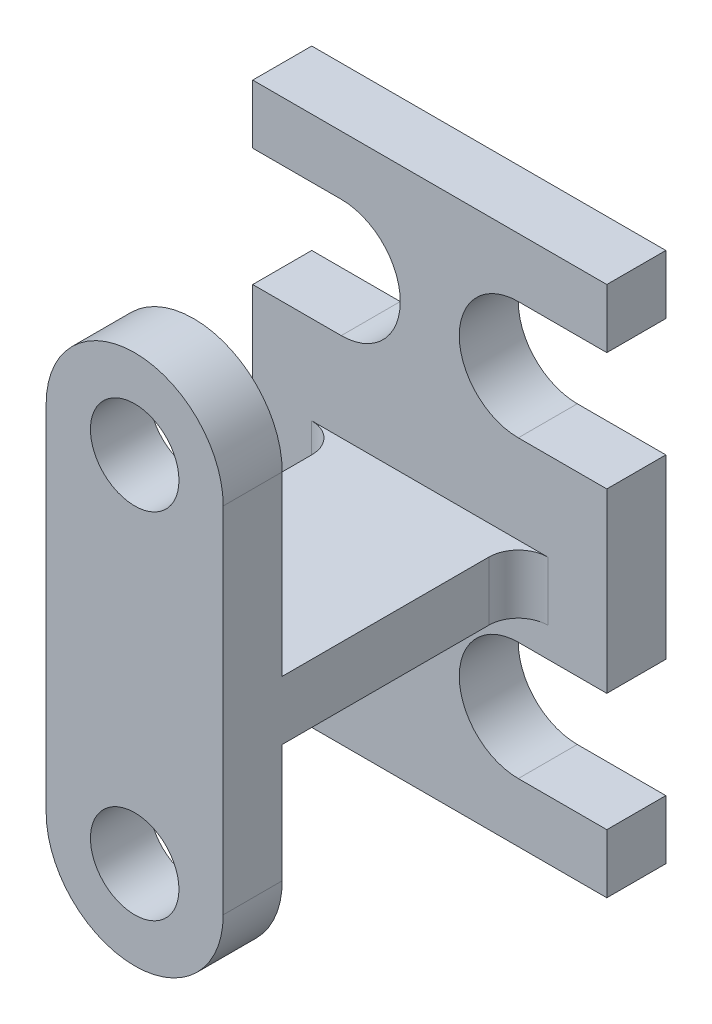
ISO-10303-21;
HEADER;
FILE_DESCRIPTION(('STEP AP214'),'2;1');
FILE_NAME('part.step','',(''),(''),'','','');
FILE_SCHEMA(('AUTOMOTIVE_DESIGN { 1 0 10303 214 1 1 1 1 }'));
ENDSEC;
DATA;
#1=APPLICATION_CONTEXT('core data for automotive mechanical design processes');
#2=APPLICATION_PROTOCOL_DEFINITION('international standard','automotive_design',2000,#1);
#3=PRODUCT_CONTEXT('',#1,'mechanical');
#4=PRODUCT('Part','Part','',(#3));
#5=PRODUCT_RELATED_PRODUCT_CATEGORY('part','',(#4));
#6=PRODUCT_DEFINITION_FORMATION('','',#4);
#7=PRODUCT_DEFINITION_CONTEXT('part definition',#1,'design');
#8=PRODUCT_DEFINITION('design','',#6,#7);
#9=PRODUCT_DEFINITION_SHAPE('','',#8);
#10=(LENGTH_UNIT() NAMED_UNIT(*) SI_UNIT(.MILLI.,.METRE.));
#11=(NAMED_UNIT(*) PLANE_ANGLE_UNIT() SI_UNIT($,.RADIAN.));
#12=(NAMED_UNIT(*) SI_UNIT($,.STERADIAN.) SOLID_ANGLE_UNIT());
#13=UNCERTAINTY_MEASURE_WITH_UNIT(LENGTH_MEASURE(1.E-05),#10,'distance_accuracy_value','');
#14=(GEOMETRIC_REPRESENTATION_CONTEXT(3) GLOBAL_UNCERTAINTY_ASSIGNED_CONTEXT((#13)) GLOBAL_UNIT_ASSIGNED_CONTEXT((#10,
#11,#12)) REPRESENTATION_CONTEXT('',''));
#15=CARTESIAN_POINT('',(0.,0.,0.));
#16=DIRECTION('',(0.,0.,1.));
#17=DIRECTION('',(1.,0.,0.));
#18=AXIS2_PLACEMENT_3D('',#15,#16,#17);
#19=CARTESIAN_POINT('',(0.,0.,0.));
#20=DIRECTION('',(0.,0.,1.));
#21=DIRECTION('',(1.,0.,0.));
#22=AXIS2_PLACEMENT_3D('',#19,#20,#21);
#23=PLANE('',#22);
#24=DIRECTION('',(1.,0.,0.));
#25=VECTOR('',#24,1.);
#26=CARTESIAN_POINT('',(-1.5,-3.5,0.));
#27=LINE('',#26,#25);
#28=CARTESIAN_POINT('',(-3.,-3.5,0.));
#29=VERTEX_POINT('',#28);
#30=CARTESIAN_POINT('',(-1.5,-3.5,0.));
#31=VERTEX_POINT('',#30);
#32=EDGE_CURVE('E327',#29,#31,#27,.T.);
#33=ORIENTED_EDGE('',*,*,#32,.F.);
#34=DIRECTION('',(0.,-1.,0.));
#35=VECTOR('',#34,1.);
#36=CARTESIAN_POINT('',(-3.,3.,0.));
#37=LINE('',#36,#35);
#38=CARTESIAN_POINT('',(-3.,-4.5,0.));
#39=VERTEX_POINT('',#38);
#40=EDGE_CURVE('E435',#29,#39,#37,.T.);
#41=ORIENTED_EDGE('',*,*,#40,.T.);
#42=DIRECTION('',(-1.,0.,0.));
#43=VECTOR('',#42,1.);
#44=CARTESIAN_POINT('',(-3.,-4.5,0.));
#45=LINE('',#44,#43);
#46=CARTESIAN_POINT('',(3.,-4.5,0.));
#47=VERTEX_POINT('',#46);
#48=EDGE_CURVE('E405',#47,#39,#45,.T.);
#49=ORIENTED_EDGE('',*,*,#48,.F.);
#50=DIRECTION('',(0.,1.,0.));
#51=VECTOR('',#50,1.);
#52=CARTESIAN_POINT('',(3.,3.,0.));
#53=LINE('',#52,#51);
#54=CARTESIAN_POINT('',(3.,-3.5,0.));
#55=VERTEX_POINT('',#54);
#56=EDGE_CURVE('E429',#47,#55,#53,.T.);
#57=ORIENTED_EDGE('',*,*,#56,.T.);
#58=DIRECTION('',(1.,0.,0.));
#59=VECTOR('',#58,1.);
#60=CARTESIAN_POINT('',(1.5,-3.5,0.));
#61=LINE('',#60,#59);
#62=CARTESIAN_POINT('',(1.5,-3.5,0.));
#63=VERTEX_POINT('',#62);
#64=EDGE_CURVE('E314',#63,#55,#61,.T.);
#65=ORIENTED_EDGE('',*,*,#64,.F.);
#66=CARTESIAN_POINT('',(1.5,-2.5,0.));
#67=DIRECTION('',(0.,0.,1.));
#68=DIRECTION('',(1.,0.,0.));
#69=AXIS2_PLACEMENT_3D('',#66,#67,#68);
#70=CIRCLE('',#69,1.);
#71=CARTESIAN_POINT('',(1.5,-1.5,0.));
#72=VERTEX_POINT('',#71);
#73=EDGE_CURVE('E311',#72,#63,#70,.T.);
#74=ORIENTED_EDGE('',*,*,#73,.F.);
#75=DIRECTION('',(-1.,0.,0.));
#76=VECTOR('',#75,1.);
#77=CARTESIAN_POINT('',(1.5,-1.5,0.));
#78=LINE('',#77,#76);
#79=CARTESIAN_POINT('',(3.,-1.5,0.));
#80=VERTEX_POINT('',#79);
#81=EDGE_CURVE('E307',#80,#72,#78,.T.);
#82=ORIENTED_EDGE('',*,*,#81,.F.);
#83=CARTESIAN_POINT('',(3.,1.5,0.));
#84=VERTEX_POINT('',#83);
#85=EDGE_CURVE('E433',#80,#84,#53,.T.);
#86=ORIENTED_EDGE('',*,*,#85,.T.);
#87=DIRECTION('',(1.,0.,0.));
#88=VECTOR('',#87,1.);
#89=CARTESIAN_POINT('',(1.5,1.5,0.));
#90=LINE('',#89,#88);
#91=CARTESIAN_POINT('',(1.5,1.5,0.));
#92=VERTEX_POINT('',#91);
#93=EDGE_CURVE('E292',#92,#84,#90,.T.);
#94=ORIENTED_EDGE('',*,*,#93,.F.);
#95=CARTESIAN_POINT('',(1.5,2.5,0.));
#96=DIRECTION('',(0.,0.,1.));
#97=DIRECTION('',(-1.,0.,0.));
#98=AXIS2_PLACEMENT_3D('',#95,#96,#97);
#99=CIRCLE('',#98,1.);
#100=CARTESIAN_POINT('',(1.5,3.5,0.));
#101=VERTEX_POINT('',#100);
#102=EDGE_CURVE('E287',#101,#92,#99,.T.);
#103=ORIENTED_EDGE('',*,*,#102,.F.);
#104=DIRECTION('',(-1.,0.,0.));
#105=VECTOR('',#104,1.);
#106=CARTESIAN_POINT('',(1.5,3.5,0.));
#107=LINE('',#106,#105);
#108=CARTESIAN_POINT('',(3.,3.5,0.));
#109=VERTEX_POINT('',#108);
#110=EDGE_CURVE('E294',#109,#101,#107,.T.);
#111=ORIENTED_EDGE('',*,*,#110,.F.);
#112=CARTESIAN_POINT('',(3.,4.5,0.));
#113=VERTEX_POINT('',#112);
#114=EDGE_CURVE('E416',#109,#113,#53,.T.);
#115=ORIENTED_EDGE('',*,*,#114,.T.);
#116=DIRECTION('',(1.,0.,0.));
#117=VECTOR('',#116,1.);
#118=CARTESIAN_POINT('',(-3.,4.5,0.));
#119=LINE('',#118,#117);
#120=CARTESIAN_POINT('',(-3.,4.5,0.));
#121=VERTEX_POINT('',#120);
#122=EDGE_CURVE('E409',#121,#113,#119,.T.);
#123=ORIENTED_EDGE('',*,*,#122,.F.);
#124=CARTESIAN_POINT('',(-3.,3.5,0.));
#125=VERTEX_POINT('',#124);
#126=EDGE_CURVE('E432',#121,#125,#37,.T.);
#127=ORIENTED_EDGE('',*,*,#126,.T.);
#128=DIRECTION('',(-1.,0.,0.));
#129=VECTOR('',#128,1.);
#130=CARTESIAN_POINT('',(-1.5,3.5,0.));
#131=LINE('',#130,#129);
#132=CARTESIAN_POINT('',(-1.5,3.5,0.));
#133=VERTEX_POINT('',#132);
#134=EDGE_CURVE('E345',#133,#125,#131,.T.);
#135=ORIENTED_EDGE('',*,*,#134,.F.);
#136=CARTESIAN_POINT('',(-1.5,2.5,0.));
#137=DIRECTION('',(0.,0.,1.));
#138=DIRECTION('',(1.,0.,0.));
#139=AXIS2_PLACEMENT_3D('',#136,#137,#138);
#140=CIRCLE('',#139,1.);
#141=CARTESIAN_POINT('',(-1.5,1.5,0.));
#142=VERTEX_POINT('',#141);
#143=EDGE_CURVE('E301',#142,#133,#140,.T.);
#144=ORIENTED_EDGE('',*,*,#143,.F.);
#145=DIRECTION('',(1.,0.,0.));
#146=VECTOR('',#145,1.);
#147=CARTESIAN_POINT('',(-1.5,1.5,0.));
#148=LINE('',#147,#146);
#149=CARTESIAN_POINT('',(-3.,1.5,0.));
#150=VERTEX_POINT('',#149);
#151=EDGE_CURVE('E341',#150,#142,#148,.T.);
#152=ORIENTED_EDGE('',*,*,#151,.F.);
#153=CARTESIAN_POINT('',(-3.,-1.5,0.));
#154=VERTEX_POINT('',#153);
#155=EDGE_CURVE('E440',#150,#154,#37,.T.);
#156=ORIENTED_EDGE('',*,*,#155,.T.);
#157=DIRECTION('',(-1.,0.,0.));
#158=VECTOR('',#157,1.);
#159=CARTESIAN_POINT('',(-1.5,-1.5,0.));
#160=LINE('',#159,#158);
#161=CARTESIAN_POINT('',(-1.5,-1.5,0.));
#162=VERTEX_POINT('',#161);
#163=EDGE_CURVE('E330',#162,#154,#160,.T.);
#164=ORIENTED_EDGE('',*,*,#163,.F.);
#165=CARTESIAN_POINT('',(-1.5,-2.5,0.));
#166=DIRECTION('',(0.,0.,1.));
#167=DIRECTION('',(-1.,0.,0.));
#168=AXIS2_PLACEMENT_3D('',#165,#166,#167);
#169=CIRCLE('',#168,1.);
#170=EDGE_CURVE('E288',#31,#162,#169,.T.);
#171=ORIENTED_EDGE('',*,*,#170,.F.);
#172=EDGE_LOOP('',(#33,#41,#49,#57,#65,#74,#82,#86,#94,#103,#111,#115,#123,#127,#135,#144,#152,
#156,#164,#171));
#173=FACE_BOUND('',#172,.T.);
#174=DIRECTION('',(1.,0.,0.));
#175=VECTOR('',#174,1.);
#176=CARTESIAN_POINT('',(1.5,-1.,0.));
#177=LINE('',#176,#175);
#178=CARTESIAN_POINT('',(-2.,-1.,0.));
#179=VERTEX_POINT('',#178);
#180=CARTESIAN_POINT('',(2.,-1.,0.));
#181=VERTEX_POINT('',#180);
#182=EDGE_CURVE('E57',#179,#181,#177,.T.);
#183=ORIENTED_EDGE('',*,*,#182,.F.);
#184=DIRECTION('',(0.,-1.,0.));
#185=VECTOR('',#184,1.);
#186=CARTESIAN_POINT('',(-2.,0.,0.));
#187=LINE('',#186,#185);
#188=CARTESIAN_POINT('',(-2.,0.,0.));
#189=VERTEX_POINT('',#188);
#190=EDGE_CURVE('E446',#179,#189,#187,.F.);
#191=ORIENTED_EDGE('',*,*,#190,.T.);
#192=DIRECTION('',(-1.,0.,0.));
#193=VECTOR('',#192,1.);
#194=CARTESIAN_POINT('',(-1.5,0.,0.));
#195=LINE('',#194,#193);
#196=CARTESIAN_POINT('',(2.,0.,0.));
#197=VERTEX_POINT('',#196);
#198=EDGE_CURVE('E64',#197,#189,#195,.T.);
#199=ORIENTED_EDGE('',*,*,#198,.F.);
#200=DIRECTION('',(0.,1.,0.));
#201=VECTOR('',#200,1.);
#202=CARTESIAN_POINT('',(2.,0.,0.));
#203=LINE('',#202,#201);
#204=EDGE_CURVE('E439',#197,#181,#203,.F.);
#205=ORIENTED_EDGE('',*,*,#204,.T.);
#206=EDGE_LOOP('',(#183,#191,#199,#205));
#207=FACE_BOUND('',#206,.T.);
#208=ADVANCED_FACE('F41',(#173,#207),#23,.T.);
#209=CARTESIAN_POINT('',(3.,3.,-1.));
#210=DIRECTION('',(1.,0.,0.));
#211=DIRECTION('',(0.,1.,0.));
#212=AXIS2_PLACEMENT_3D('',#209,#210,#211);
#213=PLANE('',#212);
#214=DIRECTION('',(0.,0.,1.));
#215=VECTOR('',#214,1.);
#216=CARTESIAN_POINT('',(3.,-1.5,-1.5));
#217=LINE('',#216,#215);
#218=CARTESIAN_POINT('',(3.,-1.5,-1.));
#219=VERTEX_POINT('',#218);
#220=EDGE_CURVE('E291',#219,#80,#217,.T.);
#221=ORIENTED_EDGE('',*,*,#220,.F.);
#222=DIRECTION('',(0.,1.,0.));
#223=VECTOR('',#222,1.);
#224=CARTESIAN_POINT('',(3.,3.,-1.));
#225=LINE('',#224,#223);
#226=CARTESIAN_POINT('',(3.,1.5,-1.));
#227=VERTEX_POINT('',#226);
#228=EDGE_CURVE('E422',#219,#227,#225,.T.);
#229=ORIENTED_EDGE('',*,*,#228,.T.);
#230=DIRECTION('',(0.,0.,1.));
#231=VECTOR('',#230,1.);
#232=CARTESIAN_POINT('',(3.,1.5,-1.5));
#233=LINE('',#232,#231);
#234=EDGE_CURVE('E302',#227,#84,#233,.T.);
#235=ORIENTED_EDGE('',*,*,#234,.T.);
#236=ORIENTED_EDGE('',*,*,#85,.F.);
#237=EDGE_LOOP('',(#221,#229,#235,#236));
#238=FACE_BOUND('',#237,.T.);
#239=ADVANCED_FACE('F503',(#238),#213,.T.);
#240=DIRECTION('',(0.,0.,1.));
#241=VECTOR('',#240,1.);
#242=CARTESIAN_POINT('',(3.,3.5,-1.5));
#243=LINE('',#242,#241);
#244=CARTESIAN_POINT('',(3.,3.5,-1.));
#245=VERTEX_POINT('',#244);
#246=EDGE_CURVE('E305',#245,#109,#243,.T.);
#247=ORIENTED_EDGE('',*,*,#246,.F.);
#248=CARTESIAN_POINT('',(3.,4.5,-1.));
#249=VERTEX_POINT('',#248);
#250=EDGE_CURVE('E421',#245,#249,#225,.T.);
#251=ORIENTED_EDGE('',*,*,#250,.T.);
#252=DIRECTION('',(0.,0.,-1.));
#253=VECTOR('',#252,1.);
#254=CARTESIAN_POINT('',(3.,4.5,-1.));
#255=LINE('',#254,#253);
#256=EDGE_CURVE('E411',#113,#249,#255,.T.);
#257=ORIENTED_EDGE('',*,*,#256,.F.);
#258=ORIENTED_EDGE('',*,*,#114,.F.);
#259=EDGE_LOOP('',(#247,#251,#257,#258));
#260=FACE_BOUND('',#259,.T.);
#261=ADVANCED_FACE('F509',(#260),#213,.T.);
#262=CARTESIAN_POINT('',(-3.,3.,-1.));
#263=DIRECTION('',(-1.,0.,0.));
#264=DIRECTION('',(0.,-1.,0.));
#265=AXIS2_PLACEMENT_3D('',#262,#263,#264);
#266=PLANE('',#265);
#267=DIRECTION('',(0.,0.,1.));
#268=VECTOR('',#267,1.);
#269=CARTESIAN_POINT('',(-3.,-3.5,-1.5));
#270=LINE('',#269,#268);
#271=CARTESIAN_POINT('',(-3.,-3.5,-1.));
#272=VERTEX_POINT('',#271);
#273=EDGE_CURVE('E333',#272,#29,#270,.T.);
#274=ORIENTED_EDGE('',*,*,#273,.F.);
#275=DIRECTION('',(0.,-1.,0.));
#276=VECTOR('',#275,1.);
#277=CARTESIAN_POINT('',(-3.,3.,-1.));
#278=LINE('',#277,#276);
#279=CARTESIAN_POINT('',(-3.,-4.5,-1.));
#280=VERTEX_POINT('',#279);
#281=EDGE_CURVE('E423',#272,#280,#278,.T.);
#282=ORIENTED_EDGE('',*,*,#281,.T.);
#283=DIRECTION('',(0.,0.,-1.));
#284=VECTOR('',#283,1.);
#285=CARTESIAN_POINT('',(-3.,-4.5,0.));
#286=LINE('',#285,#284);
#287=EDGE_CURVE('E393',#39,#280,#286,.T.);
#288=ORIENTED_EDGE('',*,*,#287,.F.);
#289=ORIENTED_EDGE('',*,*,#40,.F.);
#290=EDGE_LOOP('',(#274,#282,#288,#289));
#291=FACE_BOUND('',#290,.T.);
#292=ADVANCED_FACE('F525',(#291),#266,.T.);
#293=DIRECTION('',(0.,0.,1.));
#294=VECTOR('',#293,1.);
#295=CARTESIAN_POINT('',(-3.,-1.5,-1.5));
#296=LINE('',#295,#294);
#297=CARTESIAN_POINT('',(-3.,-1.5,-1.));
#298=VERTEX_POINT('',#297);
#299=EDGE_CURVE('E337',#298,#154,#296,.T.);
#300=ORIENTED_EDGE('',*,*,#299,.T.);
#301=ORIENTED_EDGE('',*,*,#155,.F.);
#302=DIRECTION('',(0.,0.,1.));
#303=VECTOR('',#302,1.);
#304=CARTESIAN_POINT('',(-3.,1.5,-1.5));
#305=LINE('',#304,#303);
#306=CARTESIAN_POINT('',(-3.,1.5,-1.));
#307=VERTEX_POINT('',#306);
#308=EDGE_CURVE('E354',#307,#150,#305,.T.);
#309=ORIENTED_EDGE('',*,*,#308,.F.);
#310=EDGE_CURVE('E426',#307,#298,#278,.T.);
#311=ORIENTED_EDGE('',*,*,#310,.T.);
#312=EDGE_LOOP('',(#300,#301,#309,#311));
#313=FACE_BOUND('',#312,.T.);
#314=ADVANCED_FACE('F523',(#313),#266,.T.);
#315=DIRECTION('',(0.,0.,1.));
#316=VECTOR('',#315,1.);
#317=CARTESIAN_POINT('',(3.,-3.5,-1.5));
#318=LINE('',#317,#316);
#319=CARTESIAN_POINT('',(3.,-3.5,-1.));
#320=VERTEX_POINT('',#319);
#321=EDGE_CURVE('E316',#320,#55,#318,.T.);
#322=ORIENTED_EDGE('',*,*,#321,.T.);
#323=ORIENTED_EDGE('',*,*,#56,.F.);
#324=DIRECTION('',(0.,0.,1.));
#325=VECTOR('',#324,1.);
#326=CARTESIAN_POINT('',(3.,-4.5,0.));
#327=LINE('',#326,#325);
#328=CARTESIAN_POINT('',(3.,-4.5,-1.));
#329=VERTEX_POINT('',#328);
#330=EDGE_CURVE('E398',#329,#47,#327,.T.);
#331=ORIENTED_EDGE('',*,*,#330,.F.);
#332=EDGE_CURVE('E420',#329,#320,#225,.T.);
#333=ORIENTED_EDGE('',*,*,#332,.T.);
#334=EDGE_LOOP('',(#322,#323,#331,#333));
#335=FACE_BOUND('',#334,.T.);
#336=ADVANCED_FACE('F514',(#335),#213,.T.);
#337=DIRECTION('',(0.,0.,1.));
#338=VECTOR('',#337,1.);
#339=CARTESIAN_POINT('',(-3.,3.5,-1.5));
#340=LINE('',#339,#338);
#341=CARTESIAN_POINT('',(-3.,3.5,-1.));
#342=VERTEX_POINT('',#341);
#343=EDGE_CURVE('E355',#342,#125,#340,.T.);
#344=ORIENTED_EDGE('',*,*,#343,.T.);
#345=ORIENTED_EDGE('',*,*,#126,.F.);
#346=DIRECTION('',(0.,0.,1.));
#347=VECTOR('',#346,1.);
#348=CARTESIAN_POINT('',(-3.,4.5,-1.));
#349=LINE('',#348,#347);
#350=CARTESIAN_POINT('',(-3.,4.5,-1.));
#351=VERTEX_POINT('',#350);
#352=EDGE_CURVE('E403',#351,#121,#349,.T.);
#353=ORIENTED_EDGE('',*,*,#352,.F.);
#354=EDGE_CURVE('E425',#351,#342,#278,.T.);
#355=ORIENTED_EDGE('',*,*,#354,.T.);
#356=EDGE_LOOP('',(#344,#345,#353,#355));
#357=FACE_BOUND('',#356,.T.);
#358=ADVANCED_FACE('F516',(#357),#266,.T.);
#359=CARTESIAN_POINT('',(0.,0.,-1.));
#360=DIRECTION('',(0.,0.,1.));
#361=DIRECTION('',(1.,0.,0.));
#362=AXIS2_PLACEMENT_3D('',#359,#360,#361);
#363=PLANE('',#362);
#364=ORIENTED_EDGE('',*,*,#281,.F.);
#365=DIRECTION('',(1.,0.,0.));
#366=VECTOR('',#365,1.);
#367=CARTESIAN_POINT('',(0.,-3.5,-1.));
#368=LINE('',#367,#366);
#369=CARTESIAN_POINT('',(-1.5,-3.5,-1.));
#370=VERTEX_POINT('',#369);
#371=EDGE_CURVE('E390',#272,#370,#368,.T.);
#372=ORIENTED_EDGE('',*,*,#371,.T.);
#373=CARTESIAN_POINT('',(-1.5,-2.5,-1.));
#374=DIRECTION('',(0.,0.,1.));
#375=DIRECTION('',(1.,0.,0.));
#376=AXIS2_PLACEMENT_3D('',#373,#374,#375);
#377=CIRCLE('',#376,1.);
#378=CARTESIAN_POINT('',(-1.5,-1.5,-1.));
#379=VERTEX_POINT('',#378);
#380=EDGE_CURVE('E388',#370,#379,#377,.T.);
#381=ORIENTED_EDGE('',*,*,#380,.T.);
#382=DIRECTION('',(-1.,0.,0.));
#383=VECTOR('',#382,1.);
#384=CARTESIAN_POINT('',(0.,-1.5,-1.));
#385=LINE('',#384,#383);
#386=EDGE_CURVE('E381',#379,#298,#385,.T.);
#387=ORIENTED_EDGE('',*,*,#386,.T.);
#388=ORIENTED_EDGE('',*,*,#310,.F.);
#389=DIRECTION('',(1.,0.,0.));
#390=VECTOR('',#389,1.);
#391=CARTESIAN_POINT('',(0.,1.5,-1.));
#392=LINE('',#391,#390);
#393=CARTESIAN_POINT('',(-1.5,1.5,-1.));
#394=VERTEX_POINT('',#393);
#395=EDGE_CURVE('E359',#307,#394,#392,.T.);
#396=ORIENTED_EDGE('',*,*,#395,.T.);
#397=CARTESIAN_POINT('',(-1.5,2.5,-1.));
#398=DIRECTION('',(0.,0.,1.));
#399=DIRECTION('',(1.,0.,0.));
#400=AXIS2_PLACEMENT_3D('',#397,#398,#399);
#401=CIRCLE('',#400,1.);
#402=CARTESIAN_POINT('',(-1.5,3.5,-1.));
#403=VERTEX_POINT('',#402);
#404=EDGE_CURVE('E361',#394,#403,#401,.T.);
#405=ORIENTED_EDGE('',*,*,#404,.T.);
#406=DIRECTION('',(-1.,0.,0.));
#407=VECTOR('',#406,1.);
#408=CARTESIAN_POINT('',(0.,3.5,-1.));
#409=LINE('',#408,#407);
#410=EDGE_CURVE('E349',#403,#342,#409,.T.);
#411=ORIENTED_EDGE('',*,*,#410,.T.);
#412=ORIENTED_EDGE('',*,*,#354,.F.);
#413=DIRECTION('',(-1.,0.,0.));
#414=VECTOR('',#413,1.);
#415=CARTESIAN_POINT('',(-3.,4.5,-1.));
#416=LINE('',#415,#414);
#417=EDGE_CURVE('E412',#249,#351,#416,.T.);
#418=ORIENTED_EDGE('',*,*,#417,.F.);
#419=ORIENTED_EDGE('',*,*,#250,.F.);
#420=DIRECTION('',(-1.,0.,0.));
#421=VECTOR('',#420,1.);
#422=CARTESIAN_POINT('',(0.,3.5,-1.));
#423=LINE('',#422,#421);
#424=CARTESIAN_POINT('',(1.5,3.5,-1.));
#425=VERTEX_POINT('',#424);
#426=EDGE_CURVE('E367',#245,#425,#423,.T.);
#427=ORIENTED_EDGE('',*,*,#426,.T.);
#428=CARTESIAN_POINT('',(1.5,2.5,-1.));
#429=DIRECTION('',(0.,0.,1.));
#430=DIRECTION('',(1.,0.,0.));
#431=AXIS2_PLACEMENT_3D('',#428,#429,#430);
#432=CIRCLE('',#431,1.);
#433=CARTESIAN_POINT('',(1.5,1.5,-1.));
#434=VERTEX_POINT('',#433);
#435=EDGE_CURVE('E375',#425,#434,#432,.T.);
#436=ORIENTED_EDGE('',*,*,#435,.T.);
#437=DIRECTION('',(1.,0.,0.));
#438=VECTOR('',#437,1.);
#439=CARTESIAN_POINT('',(0.,1.5,-1.));
#440=LINE('',#439,#438);
#441=EDGE_CURVE('E366',#434,#227,#440,.T.);
#442=ORIENTED_EDGE('',*,*,#441,.T.);
#443=ORIENTED_EDGE('',*,*,#228,.F.);
#444=DIRECTION('',(-1.,0.,0.));
#445=VECTOR('',#444,1.);
#446=CARTESIAN_POINT('',(0.,-1.5,-1.));
#447=LINE('',#446,#445);
#448=CARTESIAN_POINT('',(1.5,-1.5,-1.));
#449=VERTEX_POINT('',#448);
#450=EDGE_CURVE('E382',#219,#449,#447,.T.);
#451=ORIENTED_EDGE('',*,*,#450,.T.);
#452=CARTESIAN_POINT('',(1.5,-2.5,-1.));
#453=DIRECTION('',(0.,0.,1.));
#454=DIRECTION('',(1.,0.,0.));
#455=AXIS2_PLACEMENT_3D('',#452,#453,#454);
#456=CIRCLE('',#455,1.);
#457=CARTESIAN_POINT('',(1.5,-3.5,-1.));
#458=VERTEX_POINT('',#457);
#459=EDGE_CURVE('E374',#449,#458,#456,.T.);
#460=ORIENTED_EDGE('',*,*,#459,.T.);
#461=DIRECTION('',(1.,0.,0.));
#462=VECTOR('',#461,1.);
#463=CARTESIAN_POINT('',(0.,-3.5,-1.));
#464=LINE('',#463,#462);
#465=EDGE_CURVE('E377',#458,#320,#464,.T.);
#466=ORIENTED_EDGE('',*,*,#465,.T.);
#467=ORIENTED_EDGE('',*,*,#332,.F.);
#468=DIRECTION('',(1.,0.,0.));
#469=VECTOR('',#468,1.);
#470=CARTESIAN_POINT('',(-3.,-4.5,-1.));
#471=LINE('',#470,#469);
#472=EDGE_CURVE('E399',#280,#329,#471,.T.);
#473=ORIENTED_EDGE('',*,*,#472,.F.);
#474=EDGE_LOOP('',(#364,#372,#381,#387,#388,#396,#405,#411,#412,#418,#419,#427,#436,#442,#443,
#451,#460,#466,#467,#473));
#475=FACE_BOUND('',#474,.T.);
#476=ADVANCED_FACE('F520',(#475),#363,.F.);
#477=CARTESIAN_POINT('',(0.,4.5,0.));
#478=DIRECTION('',(0.,1.,0.));
#479=DIRECTION('',(0.,0.,1.));
#480=AXIS2_PLACEMENT_3D('',#477,#478,#479);
#481=PLANE('',#480);
#482=ORIENTED_EDGE('',*,*,#352,.T.);
#483=ORIENTED_EDGE('',*,*,#122,.T.);
#484=ORIENTED_EDGE('',*,*,#256,.T.);
#485=ORIENTED_EDGE('',*,*,#417,.T.);
#486=EDGE_LOOP('',(#482,#483,#484,#485));
#487=FACE_BOUND('',#486,.T.);
#488=ADVANCED_FACE('F587',(#487),#481,.T.);
#489=CARTESIAN_POINT('',(0.,-4.5,0.));
#490=DIRECTION('',(0.,-1.,0.));
#491=DIRECTION('',(0.,0.,-1.));
#492=AXIS2_PLACEMENT_3D('',#489,#490,#491);
#493=PLANE('',#492);
#494=ORIENTED_EDGE('',*,*,#287,.T.);
#495=ORIENTED_EDGE('',*,*,#472,.T.);
#496=ORIENTED_EDGE('',*,*,#330,.T.);
#497=ORIENTED_EDGE('',*,*,#48,.T.);
#498=EDGE_LOOP('',(#494,#495,#496,#497));
#499=FACE_BOUND('',#498,.T.);
#500=ADVANCED_FACE('F586',(#499),#493,.T.);
#501=CARTESIAN_POINT('',(-1.5,2.5,-1.5));
#502=DIRECTION('',(0.,0.,1.));
#503=DIRECTION('',(1.,0.,0.));
#504=AXIS2_PLACEMENT_3D('',#501,#502,#503);
#505=CYLINDRICAL_SURFACE('',#504,1.);
#506=DIRECTION('',(0.,0.,1.));
#507=VECTOR('',#506,1.);
#508=CARTESIAN_POINT('',(-1.5,1.5,-1.5));
#509=LINE('',#508,#507);
#510=EDGE_CURVE('E348',#394,#142,#509,.T.);
#511=ORIENTED_EDGE('',*,*,#510,.T.);
#512=ORIENTED_EDGE('',*,*,#143,.T.);
#513=DIRECTION('',(0.,0.,1.));
#514=VECTOR('',#513,1.);
#515=CARTESIAN_POINT('',(-1.5,3.5,-1.5));
#516=LINE('',#515,#514);
#517=EDGE_CURVE('E350',#403,#133,#516,.T.);
#518=ORIENTED_EDGE('',*,*,#517,.F.);
#519=ORIENTED_EDGE('',*,*,#404,.F.);
#520=EDGE_LOOP('',(#511,#512,#518,#519));
#521=FACE_BOUND('',#520,.T.);
#522=ADVANCED_FACE('F576',(#521),#505,.F.);
#523=CARTESIAN_POINT('',(-1.5,1.5,-1.5));
#524=DIRECTION('',(0.,-1.,0.));
#525=DIRECTION('',(1.,0.,0.));
#526=AXIS2_PLACEMENT_3D('',#523,#524,#525);
#527=PLANE('',#526);
#528=ORIENTED_EDGE('',*,*,#308,.T.);
#529=ORIENTED_EDGE('',*,*,#151,.T.);
#530=ORIENTED_EDGE('',*,*,#510,.F.);
#531=ORIENTED_EDGE('',*,*,#395,.F.);
#532=EDGE_LOOP('',(#528,#529,#530,#531));
#533=FACE_BOUND('',#532,.T.);
#534=ADVANCED_FACE('F577',(#533),#527,.F.);
#535=CARTESIAN_POINT('',(-1.5,3.5,-1.5));
#536=DIRECTION('',(0.,1.,0.));
#537=DIRECTION('',(-1.,0.,0.));
#538=AXIS2_PLACEMENT_3D('',#535,#536,#537);
#539=PLANE('',#538);
#540=ORIENTED_EDGE('',*,*,#517,.T.);
#541=ORIENTED_EDGE('',*,*,#134,.T.);
#542=ORIENTED_EDGE('',*,*,#343,.F.);
#543=ORIENTED_EDGE('',*,*,#410,.F.);
#544=EDGE_LOOP('',(#540,#541,#542,#543));
#545=FACE_BOUND('',#544,.T.);
#546=ADVANCED_FACE('F551',(#545),#539,.F.);
#547=CARTESIAN_POINT('',(1.5,2.5,-1.5));
#548=DIRECTION('',(0.,0.,1.));
#549=DIRECTION('',(1.,0.,0.));
#550=AXIS2_PLACEMENT_3D('',#547,#548,#549);
#551=CYLINDRICAL_SURFACE('',#550,1.);
#552=DIRECTION('',(0.,0.,1.));
#553=VECTOR('',#552,1.);
#554=CARTESIAN_POINT('',(1.5,3.5,-1.5));
#555=LINE('',#554,#553);
#556=EDGE_CURVE('E299',#425,#101,#555,.T.);
#557=ORIENTED_EDGE('',*,*,#556,.T.);
#558=ORIENTED_EDGE('',*,*,#102,.T.);
#559=DIRECTION('',(0.,0.,1.));
#560=VECTOR('',#559,1.);
#561=CARTESIAN_POINT('',(1.5,1.5,-1.5));
#562=LINE('',#561,#560);
#563=EDGE_CURVE('E296',#434,#92,#562,.T.);
#564=ORIENTED_EDGE('',*,*,#563,.F.);
#565=ORIENTED_EDGE('',*,*,#435,.F.);
#566=EDGE_LOOP('',(#557,#558,#564,#565));
#567=FACE_BOUND('',#566,.T.);
#568=ADVANCED_FACE('F544',(#567),#551,.F.);
#569=CARTESIAN_POINT('',(1.5,3.5,-1.5));
#570=DIRECTION('',(0.,1.,0.));
#571=DIRECTION('',(-1.,0.,0.));
#572=AXIS2_PLACEMENT_3D('',#569,#570,#571);
#573=PLANE('',#572);
#574=ORIENTED_EDGE('',*,*,#246,.T.);
#575=ORIENTED_EDGE('',*,*,#110,.T.);
#576=ORIENTED_EDGE('',*,*,#556,.F.);
#577=ORIENTED_EDGE('',*,*,#426,.F.);
#578=EDGE_LOOP('',(#574,#575,#576,#577));
#579=FACE_BOUND('',#578,.T.);
#580=ADVANCED_FACE('F541',(#579),#573,.F.);
#581=CARTESIAN_POINT('',(1.5,1.5,-1.5));
#582=DIRECTION('',(0.,-1.,0.));
#583=DIRECTION('',(1.,0.,0.));
#584=AXIS2_PLACEMENT_3D('',#581,#582,#583);
#585=PLANE('',#584);
#586=ORIENTED_EDGE('',*,*,#563,.T.);
#587=ORIENTED_EDGE('',*,*,#93,.T.);
#588=ORIENTED_EDGE('',*,*,#234,.F.);
#589=ORIENTED_EDGE('',*,*,#441,.F.);
#590=EDGE_LOOP('',(#586,#587,#588,#589));
#591=FACE_BOUND('',#590,.T.);
#592=ADVANCED_FACE('F542',(#591),#585,.F.);
#593=CARTESIAN_POINT('',(1.5,-1.5,-1.5));
#594=DIRECTION('',(0.,1.,0.));
#595=DIRECTION('',(-1.,0.,0.));
#596=AXIS2_PLACEMENT_3D('',#593,#594,#595);
#597=PLANE('',#596);
#598=ORIENTED_EDGE('',*,*,#220,.T.);
#599=ORIENTED_EDGE('',*,*,#81,.T.);
#600=DIRECTION('',(0.,0.,1.));
#601=VECTOR('',#600,1.);
#602=CARTESIAN_POINT('',(1.5,-1.5,-1.5));
#603=LINE('',#602,#601);
#604=EDGE_CURVE('E320',#449,#72,#603,.T.);
#605=ORIENTED_EDGE('',*,*,#604,.F.);
#606=ORIENTED_EDGE('',*,*,#450,.F.);
#607=EDGE_LOOP('',(#598,#599,#605,#606));
#608=FACE_BOUND('',#607,.T.);
#609=ADVANCED_FACE('F548',(#608),#597,.F.);
#610=CARTESIAN_POINT('',(1.5,-3.5,-1.5));
#611=DIRECTION('',(0.,-1.,0.));
#612=DIRECTION('',(1.,0.,0.));
#613=AXIS2_PLACEMENT_3D('',#610,#611,#612);
#614=PLANE('',#613);
#615=DIRECTION('',(0.,0.,1.));
#616=VECTOR('',#615,1.);
#617=CARTESIAN_POINT('',(1.5,-3.5,-1.5));
#618=LINE('',#617,#616);
#619=EDGE_CURVE('E325',#458,#63,#618,.T.);
#620=ORIENTED_EDGE('',*,*,#619,.T.);
#621=ORIENTED_EDGE('',*,*,#64,.T.);
#622=ORIENTED_EDGE('',*,*,#321,.F.);
#623=ORIENTED_EDGE('',*,*,#465,.F.);
#624=EDGE_LOOP('',(#620,#621,#622,#623));
#625=FACE_BOUND('',#624,.T.);
#626=ADVANCED_FACE('F554',(#625),#614,.F.);
#627=CARTESIAN_POINT('',(1.5,-2.5,-1.5));
#628=DIRECTION('',(0.,0.,1.));
#629=DIRECTION('',(1.,0.,0.));
#630=AXIS2_PLACEMENT_3D('',#627,#628,#629);
#631=CYLINDRICAL_SURFACE('',#630,1.);
#632=ORIENTED_EDGE('',*,*,#604,.T.);
#633=ORIENTED_EDGE('',*,*,#73,.T.);
#634=ORIENTED_EDGE('',*,*,#619,.F.);
#635=ORIENTED_EDGE('',*,*,#459,.F.);
#636=EDGE_LOOP('',(#632,#633,#634,#635));
#637=FACE_BOUND('',#636,.T.);
#638=ADVANCED_FACE('F556',(#637),#631,.F.);
#639=CARTESIAN_POINT('',(-1.5,-2.5,-1.5));
#640=DIRECTION('',(0.,0.,1.));
#641=DIRECTION('',(1.,0.,0.));
#642=AXIS2_PLACEMENT_3D('',#639,#640,#641);
#643=CYLINDRICAL_SURFACE('',#642,1.);
#644=DIRECTION('',(0.,0.,1.));
#645=VECTOR('',#644,1.);
#646=CARTESIAN_POINT('',(-1.5,-3.5,-1.5));
#647=LINE('',#646,#645);
#648=EDGE_CURVE('E315',#370,#31,#647,.T.);
#649=ORIENTED_EDGE('',*,*,#648,.T.);
#650=ORIENTED_EDGE('',*,*,#170,.T.);
#651=DIRECTION('',(0.,0.,1.));
#652=VECTOR('',#651,1.);
#653=CARTESIAN_POINT('',(-1.5,-1.5,-1.5));
#654=LINE('',#653,#652);
#655=EDGE_CURVE('E331',#379,#162,#654,.T.);
#656=ORIENTED_EDGE('',*,*,#655,.F.);
#657=ORIENTED_EDGE('',*,*,#380,.F.);
#658=EDGE_LOOP('',(#649,#650,#656,#657));
#659=FACE_BOUND('',#658,.T.);
#660=ADVANCED_FACE('F565',(#659),#643,.F.);
#661=CARTESIAN_POINT('',(-1.5,-3.5,-1.5));
#662=DIRECTION('',(0.,-1.,0.));
#663=DIRECTION('',(1.,0.,0.));
#664=AXIS2_PLACEMENT_3D('',#661,#662,#663);
#665=PLANE('',#664);
#666=ORIENTED_EDGE('',*,*,#273,.T.);
#667=ORIENTED_EDGE('',*,*,#32,.T.);
#668=ORIENTED_EDGE('',*,*,#648,.F.);
#669=ORIENTED_EDGE('',*,*,#371,.F.);
#670=EDGE_LOOP('',(#666,#667,#668,#669));
#671=FACE_BOUND('',#670,.T.);
#672=ADVANCED_FACE('F570',(#671),#665,.F.);
#673=CARTESIAN_POINT('',(-1.5,-1.5,-1.5));
#674=DIRECTION('',(0.,1.,0.));
#675=DIRECTION('',(-1.,0.,0.));
#676=AXIS2_PLACEMENT_3D('',#673,#674,#675);
#677=PLANE('',#676);
#678=ORIENTED_EDGE('',*,*,#655,.T.);
#679=ORIENTED_EDGE('',*,*,#163,.T.);
#680=ORIENTED_EDGE('',*,*,#299,.F.);
#681=ORIENTED_EDGE('',*,*,#386,.F.);
#682=EDGE_LOOP('',(#678,#679,#680,#681));
#683=FACE_BOUND('',#682,.T.);
#684=ADVANCED_FACE('F538',(#683),#677,.F.);
#685=CARTESIAN_POINT('',(1.5,-1.,4.));
#686=DIRECTION('',(0.,1.,0.));
#687=DIRECTION('',(0.,0.,1.));
#688=AXIS2_PLACEMENT_3D('',#685,#686,#687);
#689=PLANE('',#688);
#690=ORIENTED_EDGE('',*,*,#182,.T.);
#691=CARTESIAN_POINT('',(2.,-1.,0.5));
#692=DIRECTION('',(0.,1.,0.));
#693=DIRECTION('',(0.,0.,1.));
#694=AXIS2_PLACEMENT_3D('',#691,#692,#693);
#695=CIRCLE('',#694,0.5);
#696=CARTESIAN_POINT('',(1.5,-1.,0.5));
#697=VERTEX_POINT('',#696);
#698=EDGE_CURVE('E443',#181,#697,#695,.T.);
#699=ORIENTED_EDGE('',*,*,#698,.T.);
#700=DIRECTION('',(0.,0.,-1.));
#701=VECTOR('',#700,1.);
#702=CARTESIAN_POINT('',(1.5,-1.,4.));
#703=LINE('',#702,#701);
#704=CARTESIAN_POINT('',(1.5,-1.,4.));
#705=VERTEX_POINT('',#704);
#706=EDGE_CURVE('E289',#705,#697,#703,.T.);
#707=ORIENTED_EDGE('',*,*,#706,.F.);
#708=DIRECTION('',(1.,0.,0.));
#709=VECTOR('',#708,1.);
#710=CARTESIAN_POINT('',(1.5,-1.,4.));
#711=LINE('',#710,#709);
#712=CARTESIAN_POINT('',(-1.5,-1.,4.));
#713=VERTEX_POINT('',#712);
#714=EDGE_CURVE('E272',#713,#705,#711,.T.);
#715=ORIENTED_EDGE('',*,*,#714,.F.);
#716=DIRECTION('',(0.,0.,-1.));
#717=VECTOR('',#716,1.);
#718=CARTESIAN_POINT('',(-1.5,-1.,4.));
#719=LINE('',#718,#717);
#720=CARTESIAN_POINT('',(-1.5,-1.,0.5));
#721=VERTEX_POINT('',#720);
#722=EDGE_CURVE('E277',#713,#721,#719,.T.);
#723=ORIENTED_EDGE('',*,*,#722,.T.);
#724=CARTESIAN_POINT('',(-2.,-1.,0.5));
#725=DIRECTION('',(0.,1.,0.));
#726=DIRECTION('',(0.,0.,1.));
#727=AXIS2_PLACEMENT_3D('',#724,#725,#726);
#728=CIRCLE('',#727,0.5);
#729=EDGE_CURVE('E47',#721,#179,#728,.T.);
#730=ORIENTED_EDGE('',*,*,#729,.T.);
#731=EDGE_LOOP('',(#690,#699,#707,#715,#723,#730));
#732=FACE_BOUND('',#731,.T.);
#733=ADVANCED_FACE('F455',(#732),#689,.F.);
#734=CARTESIAN_POINT('',(1.5,0.,4.));
#735=DIRECTION('',(-1.,0.,0.));
#736=DIRECTION('',(0.,0.,1.));
#737=AXIS2_PLACEMENT_3D('',#734,#735,#736);
#738=PLANE('',#737);
#739=ORIENTED_EDGE('',*,*,#706,.T.);
#740=DIRECTION('',(0.,1.,0.));
#741=VECTOR('',#740,1.);
#742=CARTESIAN_POINT('',(1.5,0.,0.5));
#743=LINE('',#742,#741);
#744=CARTESIAN_POINT('',(1.5,0.,0.5));
#745=VERTEX_POINT('',#744);
#746=EDGE_CURVE('E430',#697,#745,#743,.T.);
#747=ORIENTED_EDGE('',*,*,#746,.T.);
#748=DIRECTION('',(0.,0.,-1.));
#749=VECTOR('',#748,1.);
#750=CARTESIAN_POINT('',(1.5,0.,4.));
#751=LINE('',#750,#749);
#752=CARTESIAN_POINT('',(1.5,0.,4.));
#753=VERTEX_POINT('',#752);
#754=EDGE_CURVE('E283',#753,#745,#751,.T.);
#755=ORIENTED_EDGE('',*,*,#754,.F.);
#756=DIRECTION('',(0.,1.,0.));
#757=VECTOR('',#756,1.);
#758=CARTESIAN_POINT('',(1.5,3.,4.));
#759=LINE('',#758,#757);
#760=CARTESIAN_POINT('',(1.5,3.,4.));
#761=VERTEX_POINT('',#760);
#762=EDGE_CURVE('E475',#753,#761,#759,.T.);
#763=ORIENTED_EDGE('',*,*,#762,.T.);
#764=DIRECTION('',(0.,0.,-1.));
#765=VECTOR('',#764,1.);
#766=CARTESIAN_POINT('',(1.5,3.,5.));
#767=LINE('',#766,#765);
#768=CARTESIAN_POINT('',(1.5,3.,5.));
#769=VERTEX_POINT('',#768);
#770=EDGE_CURVE('E478',#769,#761,#767,.T.);
#771=ORIENTED_EDGE('',*,*,#770,.F.);
#772=DIRECTION('',(0.,1.,0.));
#773=VECTOR('',#772,1.);
#774=CARTESIAN_POINT('',(1.5,3.,5.));
#775=LINE('',#774,#773);
#776=CARTESIAN_POINT('',(1.5,-3.,5.));
#777=VERTEX_POINT('',#776);
#778=EDGE_CURVE('E257',#777,#769,#775,.T.);
#779=ORIENTED_EDGE('',*,*,#778,.F.);
#780=DIRECTION('',(0.,0.,-1.));
#781=VECTOR('',#780,1.);
#782=CARTESIAN_POINT('',(1.5,-3.,5.));
#783=LINE('',#782,#781);
#784=CARTESIAN_POINT('',(1.5,-3.,4.));
#785=VERTEX_POINT('',#784);
#786=EDGE_CURVE('E266',#777,#785,#783,.T.);
#787=ORIENTED_EDGE('',*,*,#786,.T.);
#788=EDGE_CURVE('E258',#785,#705,#759,.T.);
#789=ORIENTED_EDGE('',*,*,#788,.T.);
#790=EDGE_LOOP('',(#739,#747,#755,#763,#771,#779,#787,#789));
#791=FACE_BOUND('',#790,.T.);
#792=ADVANCED_FACE('F467',(#791),#738,.F.);
#793=CARTESIAN_POINT('',(-1.5,0.,4.));
#794=DIRECTION('',(0.,-1.,0.));
#795=DIRECTION('',(0.,0.,-1.));
#796=AXIS2_PLACEMENT_3D('',#793,#794,#795);
#797=PLANE('',#796);
#798=ORIENTED_EDGE('',*,*,#198,.T.);
#799=CARTESIAN_POINT('',(-2.,0.,0.5));
#800=DIRECTION('',(0.,-1.,0.));
#801=DIRECTION('',(0.,0.,-1.));
#802=AXIS2_PLACEMENT_3D('',#799,#800,#801);
#803=CIRCLE('',#802,0.5);
#804=CARTESIAN_POINT('',(-1.5,0.,0.5));
#805=VERTEX_POINT('',#804);
#806=EDGE_CURVE('E11',#189,#805,#803,.T.);
#807=ORIENTED_EDGE('',*,*,#806,.T.);
#808=DIRECTION('',(0.,0.,-1.));
#809=VECTOR('',#808,1.);
#810=CARTESIAN_POINT('',(-1.5,0.,4.));
#811=LINE('',#810,#809);
#812=CARTESIAN_POINT('',(-1.5,0.,4.));
#813=VERTEX_POINT('',#812);
#814=EDGE_CURVE('E281',#813,#805,#811,.T.);
#815=ORIENTED_EDGE('',*,*,#814,.F.);
#816=DIRECTION('',(-1.,0.,0.));
#817=VECTOR('',#816,1.);
#818=CARTESIAN_POINT('',(-1.5,0.,4.));
#819=LINE('',#818,#817);
#820=EDGE_CURVE('E274',#753,#813,#819,.T.);
#821=ORIENTED_EDGE('',*,*,#820,.F.);
#822=ORIENTED_EDGE('',*,*,#754,.T.);
#823=CARTESIAN_POINT('',(2.,0.,0.5));
#824=DIRECTION('',(0.,-1.,0.));
#825=DIRECTION('',(0.,0.,-1.));
#826=AXIS2_PLACEMENT_3D('',#823,#824,#825);
#827=CIRCLE('',#826,0.5);
#828=EDGE_CURVE('E445',#745,#197,#827,.T.);
#829=ORIENTED_EDGE('',*,*,#828,.T.);
#830=EDGE_LOOP('',(#798,#807,#815,#821,#822,#829));
#831=FACE_BOUND('',#830,.T.);
#832=ADVANCED_FACE('F457',(#831),#797,.F.);
#833=CARTESIAN_POINT('',(-1.5,-1.,4.));
#834=DIRECTION('',(1.,0.,0.));
#835=DIRECTION('',(0.,0.,-1.));
#836=AXIS2_PLACEMENT_3D('',#833,#834,#835);
#837=PLANE('',#836);
#838=ORIENTED_EDGE('',*,*,#814,.T.);
#839=DIRECTION('',(0.,-1.,0.));
#840=VECTOR('',#839,1.);
#841=CARTESIAN_POINT('',(-1.5,-1.,0.5));
#842=LINE('',#841,#840);
#843=EDGE_CURVE('E447',#805,#721,#842,.T.);
#844=ORIENTED_EDGE('',*,*,#843,.T.);
#845=ORIENTED_EDGE('',*,*,#722,.F.);
#846=DIRECTION('',(0.,-1.,0.));
#847=VECTOR('',#846,1.);
#848=CARTESIAN_POINT('',(-1.5,3.,4.));
#849=LINE('',#848,#847);
#850=CARTESIAN_POINT('',(-1.5,-3.,4.));
#851=VERTEX_POINT('',#850);
#852=EDGE_CURVE('E481',#713,#851,#849,.T.);
#853=ORIENTED_EDGE('',*,*,#852,.T.);
#854=DIRECTION('',(0.,0.,-1.));
#855=VECTOR('',#854,1.);
#856=CARTESIAN_POINT('',(-1.5,-3.,5.));
#857=LINE('',#856,#855);
#858=CARTESIAN_POINT('',(-1.5,-3.,5.));
#859=VERTEX_POINT('',#858);
#860=EDGE_CURVE('E246',#859,#851,#857,.T.);
#861=ORIENTED_EDGE('',*,*,#860,.F.);
#862=DIRECTION('',(0.,-1.,0.));
#863=VECTOR('',#862,1.);
#864=CARTESIAN_POINT('',(-1.5,3.,5.));
#865=LINE('',#864,#863);
#866=CARTESIAN_POINT('',(-1.5,3.,5.));
#867=VERTEX_POINT('',#866);
#868=EDGE_CURVE('E240',#867,#859,#865,.T.);
#869=ORIENTED_EDGE('',*,*,#868,.F.);
#870=DIRECTION('',(0.,0.,-1.));
#871=VECTOR('',#870,1.);
#872=CARTESIAN_POINT('',(-1.5,3.,5.));
#873=LINE('',#872,#871);
#874=CARTESIAN_POINT('',(-1.5,3.,4.));
#875=VERTEX_POINT('',#874);
#876=EDGE_CURVE('E243',#867,#875,#873,.T.);
#877=ORIENTED_EDGE('',*,*,#876,.T.);
#878=EDGE_CURVE('E483',#875,#813,#849,.T.);
#879=ORIENTED_EDGE('',*,*,#878,.T.);
#880=EDGE_LOOP('',(#838,#844,#845,#853,#861,#869,#877,#879));
#881=FACE_BOUND('',#880,.T.);
#882=ADVANCED_FACE('F239',(#881),#837,.F.);
#883=CARTESIAN_POINT('',(2.,0.,0.5));
#884=DIRECTION('',(0.,1.,0.));
#885=DIRECTION('',(0.,0.,1.));
#886=AXIS2_PLACEMENT_3D('',#883,#884,#885);
#887=CYLINDRICAL_SURFACE('',#886,0.5);
#888=ORIENTED_EDGE('',*,*,#698,.F.);
#889=ORIENTED_EDGE('',*,*,#204,.F.);
#890=ORIENTED_EDGE('',*,*,#828,.F.);
#891=ORIENTED_EDGE('',*,*,#746,.F.);
#892=EDGE_LOOP('',(#888,#889,#890,#891));
#893=FACE_BOUND('',#892,.T.);
#894=ADVANCED_FACE('F465',(#893),#887,.F.);
#895=CARTESIAN_POINT('',(-2.,-1.,0.5));
#896=DIRECTION('',(0.,-1.,0.));
#897=DIRECTION('',(0.,0.,-1.));
#898=AXIS2_PLACEMENT_3D('',#895,#896,#897);
#899=CYLINDRICAL_SURFACE('',#898,0.5);
#900=ORIENTED_EDGE('',*,*,#806,.F.);
#901=ORIENTED_EDGE('',*,*,#190,.F.);
#902=ORIENTED_EDGE('',*,*,#729,.F.);
#903=ORIENTED_EDGE('',*,*,#843,.F.);
#904=EDGE_LOOP('',(#900,#901,#902,#903));
#905=FACE_BOUND('',#904,.T.);
#906=ADVANCED_FACE('F43',(#905),#899,.F.);
#907=CARTESIAN_POINT('',(0.,3.,4.));
#908=DIRECTION('',(0.,0.,1.));
#909=DIRECTION('',(1.,0.,0.));
#910=AXIS2_PLACEMENT_3D('',#907,#908,#909);
#911=PLANE('',#910);
#912=CARTESIAN_POINT('',(0.,-3.,4.));
#913=DIRECTION('',(0.,0.,1.));
#914=DIRECTION('',(1.,0.,0.));
#915=AXIS2_PLACEMENT_3D('',#912,#913,#914);
#916=CIRCLE('',#915,0.75);
#917=CARTESIAN_POINT('',(0.750000000000002,-3.,4.));
#918=VERTEX_POINT('',#917);
#919=EDGE_CURVE('E883',#918,#918,#916,.T.);
#920=ORIENTED_EDGE('',*,*,#919,.T.);
#921=EDGE_LOOP('',(#920));
#922=FACE_BOUND('',#921,.T.);
#923=ORIENTED_EDGE('',*,*,#852,.F.);
#924=ORIENTED_EDGE('',*,*,#714,.T.);
#925=ORIENTED_EDGE('',*,*,#788,.F.);
#926=CARTESIAN_POINT('',(0.,-3.,4.));
#927=DIRECTION('',(0.,0.,1.));
#928=DIRECTION('',(1.,0.,0.));
#929=AXIS2_PLACEMENT_3D('',#926,#927,#928);
#930=CIRCLE('',#929,1.5);
#931=EDGE_CURVE('E471',#851,#785,#930,.T.);
#932=ORIENTED_EDGE('',*,*,#931,.F.);
#933=EDGE_LOOP('',(#923,#924,#925,#932));
#934=FACE_BOUND('',#933,.T.);
#935=ADVANCED_FACE('F486',(#922,#934),#911,.F.);
#936=CARTESIAN_POINT('',(0.,3.,4.));
#937=DIRECTION('',(0.,0.,1.));
#938=DIRECTION('',(1.,0.,0.));
#939=AXIS2_PLACEMENT_3D('',#936,#937,#938);
#940=CIRCLE('',#939,0.75);
#941=CARTESIAN_POINT('',(0.75,3.,4.));
#942=VERTEX_POINT('',#941);
#943=EDGE_CURVE('E881',#942,#942,#940,.T.);
#944=ORIENTED_EDGE('',*,*,#943,.T.);
#945=EDGE_LOOP('',(#944));
#946=FACE_BOUND('',#945,.T.);
#947=ORIENTED_EDGE('',*,*,#762,.F.);
#948=ORIENTED_EDGE('',*,*,#820,.T.);
#949=ORIENTED_EDGE('',*,*,#878,.F.);
#950=CARTESIAN_POINT('',(0.,3.,4.));
#951=DIRECTION('',(0.,0.,1.));
#952=DIRECTION('',(1.,0.,0.));
#953=AXIS2_PLACEMENT_3D('',#950,#951,#952);
#954=CIRCLE('',#953,1.5);
#955=EDGE_CURVE('E262',#761,#875,#954,.T.);
#956=ORIENTED_EDGE('',*,*,#955,.F.);
#957=EDGE_LOOP('',(#947,#948,#949,#956));
#958=FACE_BOUND('',#957,.T.);
#959=ADVANCED_FACE('F489',(#946,#958),#911,.F.);
#960=CARTESIAN_POINT('',(0.,3.,5.));
#961=DIRECTION('',(0.,0.,1.));
#962=DIRECTION('',(1.,0.,0.));
#963=AXIS2_PLACEMENT_3D('',#960,#961,#962);
#964=PLANE('',#963);
#965=CARTESIAN_POINT('',(0.,3.,5.));
#966=DIRECTION('',(0.,0.,1.));
#967=DIRECTION('',(1.,0.,0.));
#968=AXIS2_PLACEMENT_3D('',#965,#966,#967);
#969=CIRCLE('',#968,0.75);
#970=CARTESIAN_POINT('',(0.75,3.,5.));
#971=VERTEX_POINT('',#970);
#972=EDGE_CURVE('E485',#971,#971,#969,.T.);
#973=ORIENTED_EDGE('',*,*,#972,.F.);
#974=EDGE_LOOP('',(#973));
#975=FACE_BOUND('',#974,.T.);
#976=CARTESIAN_POINT('',(0.,3.,5.));
#977=DIRECTION('',(0.,0.,1.));
#978=DIRECTION('',(1.,0.,0.));
#979=AXIS2_PLACEMENT_3D('',#976,#977,#978);
#980=CIRCLE('',#979,1.5);
#981=EDGE_CURVE('E249',#769,#867,#980,.T.);
#982=ORIENTED_EDGE('',*,*,#981,.T.);
#983=ORIENTED_EDGE('',*,*,#868,.T.);
#984=CARTESIAN_POINT('',(0.,-3.,5.));
#985=DIRECTION('',(0.,0.,1.));
#986=DIRECTION('',(1.,0.,0.));
#987=AXIS2_PLACEMENT_3D('',#984,#985,#986);
#988=CIRCLE('',#987,1.5);
#989=EDGE_CURVE('E248',#859,#777,#988,.T.);
#990=ORIENTED_EDGE('',*,*,#989,.T.);
#991=ORIENTED_EDGE('',*,*,#778,.T.);
#992=EDGE_LOOP('',(#982,#983,#990,#991));
#993=FACE_BOUND('',#992,.T.);
#994=CARTESIAN_POINT('',(0.,-3.,5.));
#995=DIRECTION('',(0.,0.,1.));
#996=DIRECTION('',(1.,0.,0.));
#997=AXIS2_PLACEMENT_3D('',#994,#995,#996);
#998=CIRCLE('',#997,0.75);
#999=CARTESIAN_POINT('',(0.750000000000002,-3.,5.));
#1000=VERTEX_POINT('',#999);
#1001=EDGE_CURVE('E880',#1000,#1000,#998,.T.);
#1002=ORIENTED_EDGE('',*,*,#1001,.F.);
#1003=EDGE_LOOP('',(#1002));
#1004=FACE_BOUND('',#1003,.T.);
#1005=ADVANCED_FACE('F254',(#975,#993,#1004),#964,.T.);
#1006=CARTESIAN_POINT('',(0.,3.,5.));
#1007=DIRECTION('',(0.,0.,-1.));
#1008=DIRECTION('',(-1.,0.,0.));
#1009=AXIS2_PLACEMENT_3D('',#1006,#1007,#1008);
#1010=CYLINDRICAL_SURFACE('',#1009,1.5);
#1011=ORIENTED_EDGE('',*,*,#955,.T.);
#1012=ORIENTED_EDGE('',*,*,#876,.F.);
#1013=ORIENTED_EDGE('',*,*,#981,.F.);
#1014=ORIENTED_EDGE('',*,*,#770,.T.);
#1015=EDGE_LOOP('',(#1011,#1012,#1013,#1014));
#1016=FACE_BOUND('',#1015,.T.);
#1017=ADVANCED_FACE('F265',(#1016),#1010,.T.);
#1018=CARTESIAN_POINT('',(0.,-3.,5.));
#1019=DIRECTION('',(0.,0.,-1.));
#1020=DIRECTION('',(-1.,0.,0.));
#1021=AXIS2_PLACEMENT_3D('',#1018,#1019,#1020);
#1022=CYLINDRICAL_SURFACE('',#1021,1.5);
#1023=ORIENTED_EDGE('',*,*,#931,.T.);
#1024=ORIENTED_EDGE('',*,*,#786,.F.);
#1025=ORIENTED_EDGE('',*,*,#989,.F.);
#1026=ORIENTED_EDGE('',*,*,#860,.T.);
#1027=EDGE_LOOP('',(#1023,#1024,#1025,#1026));
#1028=FACE_BOUND('',#1027,.T.);
#1029=ADVANCED_FACE('F487',(#1028),#1022,.T.);
#1030=CARTESIAN_POINT('',(0.,3.,5.));
#1031=DIRECTION('',(0.,0.,-1.));
#1032=DIRECTION('',(-1.,0.,0.));
#1033=AXIS2_PLACEMENT_3D('',#1030,#1031,#1032);
#1034=CYLINDRICAL_SURFACE('',#1033,0.75);
#1035=ORIENTED_EDGE('',*,*,#972,.T.);
#1036=EDGE_LOOP('',(#1035));
#1037=FACE_BOUND('',#1036,.T.);
#1038=ORIENTED_EDGE('',*,*,#943,.F.);
#1039=EDGE_LOOP('',(#1038));
#1040=FACE_BOUND('',#1039,.T.);
#1041=ADVANCED_FACE('F854',(#1037,#1040),#1034,.F.);
#1042=CARTESIAN_POINT('',(0.,-3.,5.));
#1043=DIRECTION('',(0.,0.,-1.));
#1044=DIRECTION('',(-1.,0.,0.));
#1045=AXIS2_PLACEMENT_3D('',#1042,#1043,#1044);
#1046=CYLINDRICAL_SURFACE('',#1045,0.75);
#1047=ORIENTED_EDGE('',*,*,#1001,.T.);
#1048=EDGE_LOOP('',(#1047));
#1049=FACE_BOUND('',#1048,.T.);
#1050=ORIENTED_EDGE('',*,*,#919,.F.);
#1051=EDGE_LOOP('',(#1050));
#1052=FACE_BOUND('',#1051,.T.);
#1053=ADVANCED_FACE('F856',(#1049,#1052),#1046,.F.);
#1054=CLOSED_SHELL('',(#208,#239,#261,#292,#314,#336,#358,#476,#488,#500,#522,#534,#546,#568,
#580,#592,#609,#626,#638,#660,#672,#684,#733,#792,#832,#882,#894,#906,#935,#959,#1005,#1017,
#1029,#1041,#1053));
#1055=MANIFOLD_SOLID_BREP('B2',#1054);
#1056=ADVANCED_BREP_SHAPE_REPRESENTATION('',(#18,#1055),#14);
#1057=SHAPE_DEFINITION_REPRESENTATION(#9,#1056);
ENDSEC;
END-ISO-10303-21;
